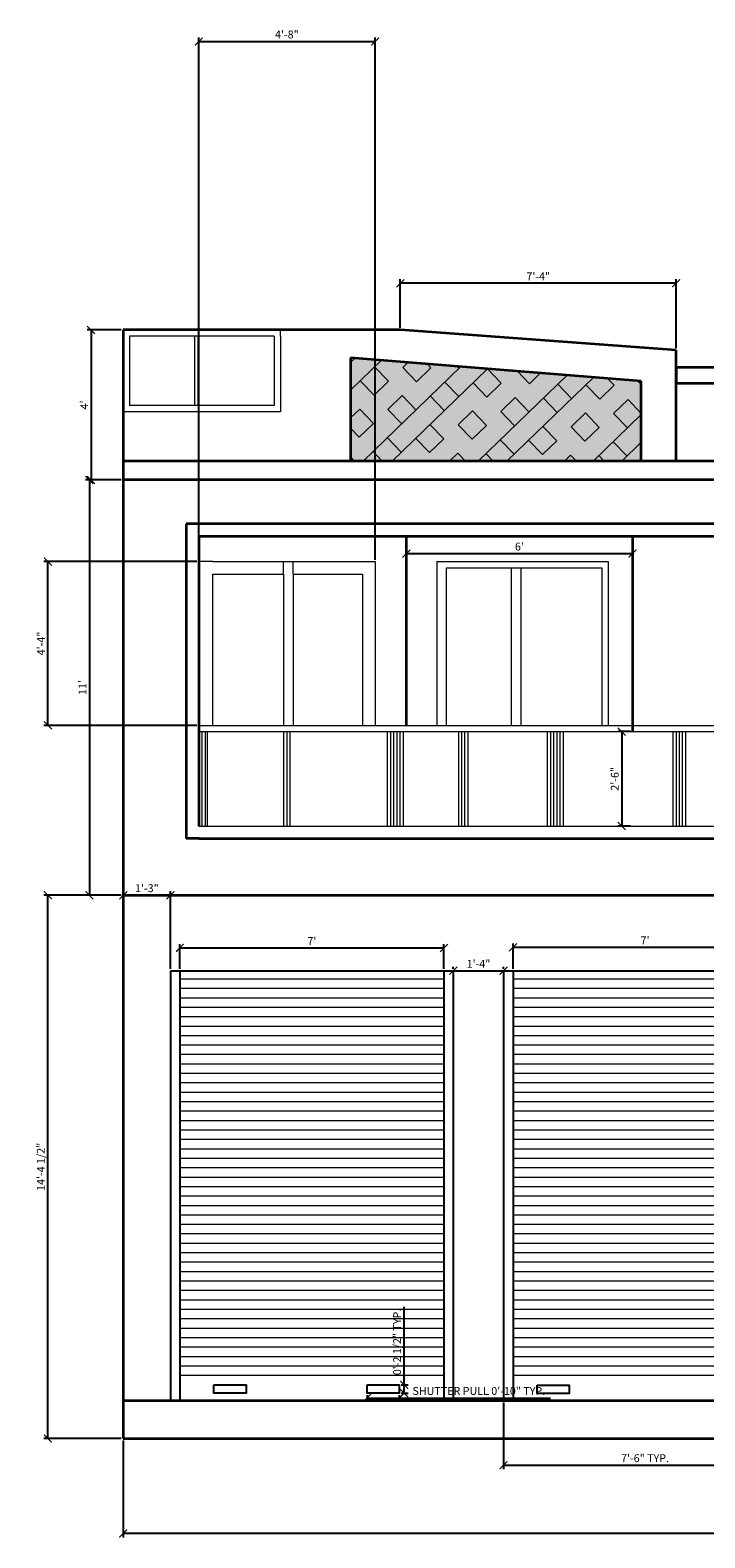
# Model space of a CAD drawing. Units: inches. Extents: x 3122 to 5933, y 1474 to 2995.
# Tile 1 of 12: x 3122 to 3337, y 1583 to 2063. Entities that reach past the tile are written whole.
import ezdxf

# ---------------------------------------------------------------- set-up
doc = ezdxf.new("R2010")
doc.units = ezdxf.units.IN
for name, color, linetype, lineweight in [('A-ANNO-DIMS', 2, 'Continuous', 18), ('A-ELEV', 7, 'Continuous', 35), ('A-ELEV-DOOR', 4, 'Continuous', 25), ('A-ELEV-GLAZ', 4, 'Continuous', 18), ('A-ELEV-PATT', 8, 'Continuous', 13), ('A-ELEV-RAIL', 7, 'Continuous', 18)]:
    doc.layers.add(name, color=color, linetype=linetype, lineweight=lineweight)
doc.styles.get("Standard").update_dxf_attribs({"font": 'arial.ttf'})
doc.dimstyles.new('ISO-25', dxfattribs={"dimtxt": 2.5, "dimasz": 2.5, "dimexe": 1.25, "dimexo": 0.625, "dimtad": 1, "dimdec": 0, "dimlunit": 3, "dimtxsty": 'Standard', "dimblk": 'ARCHTICK', "dimcen": 2.5, "dimadec": 0, "dimazin": 0, "dimtfac": 1, "dimtdec": 0, "dimtmove": 0, "dimatfit": 3, "dimfxl": 1, "dimarcsym": 0})

# ---------------------------------------------------------------- blocks, each defined once
blk = doc.blocks.new('_ArchTick')
at = {"color": 0, "linetype": 'ByBlock', "const_width": 0.15}
blk.add_lwpolyline([(-0.5, -0.5), (0.5, 0.5)], dxfattribs=at)
blk = doc.blocks.new('*D2')
at = {"layer": 'A-ANNO-DIMS', "color": 0, "lineweight": -2, "transparency": 16777216}
for p, q in [((3241.71, 1900.94), (3241.71, 1894.91)), ((3313.71, 1900.94), (3313.71, 1894.91)), ((3241.71, 1896.16), (3313.71, 1896.16))]:
    blk.add_line(p, q, dxfattribs=at)
at = {"layer": 'Defpoints', "color": 0, "transparency": 16777216}
for p in [(3241.71, 1901.56), (3313.71, 1901.56), (3313.71, 1896.16)]:
    blk.add_point(p, dxfattribs=at)
at = {"layer": 'A-ANNO-DIMS', "color": 0, "lineweight": -2, "transparency": 16777216, "xscale": 2.5, "yscale": 2.5, "zscale": 2.5, "rotation": 180}
blk.add_blockref('_ArchTick', (3241.71, 1896.16), dxfattribs=at)
at = {"layer": 'A-ANNO-DIMS', "color": 0, "lineweight": -2, "transparency": 16777216, "xscale": 2.5, "yscale": 2.5, "zscale": 2.5}
blk.add_blockref('_ArchTick', (3313.71, 1896.16), dxfattribs=at)
at = {"layer": 'A-ANNO-DIMS', "color": 0, "transparency": 16777216, "insert": (3277.71, 1898.06), "char_height": 2.5, "attachment_point": 5}
blk.add_mtext("6'", dxfattribs=at)
blk = doc.blocks.new('*D7')
at = {"layer": 'A-ANNO-DIMS', "color": 0, "lineweight": -2, "transparency": 16777216}
for p, q in [((3151.05, 1967.24), (3140.16, 1967.24)), ((3141.41, 1967.24), (3141.41, 1919.56)), ((3151.05, 1919.56), (3140.16, 1919.56))]:
    blk.add_line(p, q, dxfattribs=at)
at = {"layer": 'Defpoints', "color": 0, "transparency": 16777216}
for p in [(3151.68, 1967.24), (3141.41, 1919.56), (3151.68, 1919.56)]:
    blk.add_point(p, dxfattribs=at)
at = {"layer": 'A-ANNO-DIMS', "color": 0, "lineweight": -2, "transparency": 16777216, "xscale": 2.5, "yscale": 2.5, "zscale": 2.5}
for p, rotation in [((3141.41, 1967.24), 90), ((3141.41, 1919.56), 270)]:
    blk.add_blockref('_ArchTick', p, dxfattribs=dict(at, rotation=rotation))
at = {"layer": 'A-ANNO-DIMS', "color": 0, "transparency": 16777216, "insert": (3139.53, 1943.4), "char_height": 2.5, "attachment_point": 5, "rotation": 90}
blk.add_mtext("4'", dxfattribs=at)
blk = doc.blocks.new('*D8')
at = {"layer": 'A-ANNO-DIMS', "color": 0, "lineweight": -2, "transparency": 16777216}
for p, q in [((3151.05, 1919.56), (3139.65, 1919.56)), ((3140.9, 1919.56), (3140.9, 1787.56)), ((3151.05, 1787.56), (3139.65, 1787.56))]:
    blk.add_line(p, q, dxfattribs=at)
at = {"layer": 'Defpoints', "color": 0, "transparency": 16777216}
for p in [(3151.68, 1919.56), (3140.9, 1787.56), (3151.68, 1787.56)]:
    blk.add_point(p, dxfattribs=at)
at = {"layer": 'A-ANNO-DIMS', "color": 0, "lineweight": -2, "transparency": 16777216, "xscale": 2.5, "yscale": 2.5, "zscale": 2.5}
for p, rotation in [((3140.9, 1919.56), 90), ((3140.9, 1787.56), 270)]:
    blk.add_blockref('_ArchTick', p, dxfattribs=dict(at, rotation=rotation))
at = {"layer": 'A-ANNO-DIMS', "color": 0, "transparency": 16777216, "insert": (3139.02, 1853.56), "char_height": 2.5, "attachment_point": 5, "rotation": 90}
blk.add_mtext("11'", dxfattribs=at)
blk = doc.blocks.new('*D9')
at = {"layer": 'A-ANNO-DIMS', "color": 0, "lineweight": -2, "transparency": 16777216}
for p, q in [((3169.68, 1764.19), (3169.68, 1772.06)), ((3169.68, 1770.81), (3253.68, 1770.81)), ((3253.68, 1764.19), (3253.68, 1772.06))]:
    blk.add_line(p, q, dxfattribs=at)
at = {"layer": 'Defpoints', "color": 0, "transparency": 16777216}
for p in [(3253.68, 1770.81), (3169.68, 1763.56), (3253.68, 1763.56)]:
    blk.add_point(p, dxfattribs=at)
at = {"layer": 'A-ANNO-DIMS', "color": 0, "lineweight": -2, "transparency": 16777216, "xscale": 2.5, "yscale": 2.5, "zscale": 2.5, "rotation": 180}
blk.add_blockref('_ArchTick', (3169.68, 1770.81), dxfattribs=at)
at = {"layer": 'A-ANNO-DIMS', "color": 0, "lineweight": -2, "transparency": 16777216, "xscale": 2.5, "yscale": 2.5, "zscale": 2.5}
blk.add_blockref('_ArchTick', (3253.68, 1770.81), dxfattribs=at)
at = {"layer": 'A-ANNO-DIMS', "color": 0, "transparency": 16777216, "insert": (3211.68, 1772.68), "char_height": 2.5, "attachment_point": 5}
blk.add_mtext("7'", dxfattribs=at)
blk = doc.blocks.new('*D10')
at = {"layer": 'A-ANNO-DIMS', "color": 0, "lineweight": -2, "transparency": 16777216}
for p, q in [((3275.68, 1764.19), (3275.68, 1772.26)), ((3275.68, 1771.01), (3359.68, 1771.01)), ((3359.68, 1764.19), (3359.68, 1772.26))]:
    blk.add_line(p, q, dxfattribs=at)
at = {"layer": 'Defpoints', "color": 0, "transparency": 16777216}
for p in [(3359.68, 1771.01), (3275.68, 1763.56), (3359.68, 1763.56)]:
    blk.add_point(p, dxfattribs=at)
at = {"layer": 'A-ANNO-DIMS', "color": 0, "lineweight": -2, "transparency": 16777216, "xscale": 2.5, "yscale": 2.5, "zscale": 2.5, "rotation": 180}
blk.add_blockref('_ArchTick', (3275.68, 1771.01), dxfattribs=at)
at = {"layer": 'A-ANNO-DIMS', "color": 0, "lineweight": -2, "transparency": 16777216, "xscale": 2.5, "yscale": 2.5, "zscale": 2.5}
blk.add_blockref('_ArchTick', (3359.68, 1771.01), dxfattribs=at)
at = {"layer": 'A-ANNO-DIMS', "color": 0, "transparency": 16777216, "insert": (3317.68, 1772.89), "char_height": 2.5, "attachment_point": 5}
blk.add_mtext("7'", dxfattribs=at)
blk = doc.blocks.new('*D11')
at = {"layer": 'A-ANNO-DIMS', "color": 0, "lineweight": -2, "transparency": 16777216}
for p, q in [((3256.68, 1764.19), (3256.68, 1764.81)), ((3256.68, 1763.56), (3272.68, 1763.56)), ((3272.68, 1764.19), (3272.68, 1764.81))]:
    blk.add_line(p, q, dxfattribs=at)
at = {"layer": 'Defpoints', "color": 0, "transparency": 16777216}
for p in [(3256.68, 1763.56), (3272.68, 1763.56), (3272.68, 1763.56)]:
    blk.add_point(p, dxfattribs=at)
at = {"layer": 'A-ANNO-DIMS', "color": 0, "lineweight": -2, "transparency": 16777216, "xscale": 2.5, "yscale": 2.5, "zscale": 2.5, "rotation": 180}
blk.add_blockref('_ArchTick', (3256.68, 1763.56), dxfattribs=at)
at = {"layer": 'A-ANNO-DIMS', "color": 0, "lineweight": -2, "transparency": 16777216, "xscale": 2.5, "yscale": 2.5, "zscale": 2.5}
blk.add_blockref('_ArchTick', (3272.68, 1763.56), dxfattribs=at)
at = {"layer": 'A-ANNO-DIMS', "color": 0, "transparency": 16777216, "insert": (3264.68, 1765.44), "char_height": 2.5, "attachment_point": 5}
blk.add_mtext('1\'-4"', dxfattribs=at)
blk = doc.blocks.new('*D13')
at = {"layer": 'A-ANNO-DIMS', "color": 0, "lineweight": -2, "transparency": 16777216}
for p, q in [((3151.68, 1614.29), (3151.68, 1583.45)), ((3535.57, 1614.29), (3535.57, 1583.45)), ((3535.57, 1584.7), (3151.68, 1584.7))]:
    blk.add_line(p, q, dxfattribs=at)
at = {"layer": 'Defpoints', "color": 0, "transparency": 16777216}
for p in [(3151.68, 1614.92), (3535.57, 1614.92), (3151.68, 1584.7)]:
    blk.add_point(p, dxfattribs=at)
at = {"layer": 'A-ANNO-DIMS', "color": 0, "lineweight": -2, "transparency": 16777216, "xscale": 2.5, "yscale": 2.5, "zscale": 2.5, "rotation": 180}
blk.add_blockref('_ArchTick', (3151.68, 1584.7), dxfattribs=at)
at = {"layer": 'A-ANNO-DIMS', "color": 0, "lineweight": -2, "transparency": 16777216, "xscale": 2.5, "yscale": 2.5, "zscale": 2.5}
blk.add_blockref('_ArchTick', (3535.57, 1584.7), dxfattribs=at)
at = {"layer": 'A-ANNO-DIMS', "color": 0, "transparency": 16777216, "insert": (3343.62, 1586.6), "char_height": 2.5, "attachment_point": 5}
blk.add_mtext("32'", dxfattribs=at)
blk = doc.blocks.new('*D15')
at = {"layer": 'A-ANNO-DIMS', "color": 0, "lineweight": -2, "transparency": 16777216}
for p, q in [((3239.82, 1967.87), (3239.82, 1983.33)), ((3327.58, 1982.08), (3239.82, 1982.08)), ((3327.58, 1961.4), (3327.58, 1983.33))]:
    blk.add_line(p, q, dxfattribs=at)
at = {"layer": 'Defpoints', "color": 0, "transparency": 16777216}
for p in [(3239.82, 1982.08), (3239.82, 1967.24), (3327.58, 1960.78)]:
    blk.add_point(p, dxfattribs=at)
at = {"layer": 'A-ANNO-DIMS', "color": 0, "lineweight": -2, "transparency": 16777216, "xscale": 2.5, "yscale": 2.5, "zscale": 2.5, "rotation": 180}
blk.add_blockref('_ArchTick', (3239.82, 1982.08), dxfattribs=at)
at = {"layer": 'A-ANNO-DIMS', "color": 0, "lineweight": -2, "transparency": 16777216, "xscale": 2.5, "yscale": 2.5, "zscale": 2.5}
blk.add_blockref('_ArchTick', (3327.58, 1982.08), dxfattribs=at)
at = {"layer": 'A-ANNO-DIMS', "color": 0, "transparency": 16777216, "insert": (3283.7, 1983.96), "char_height": 2.5, "attachment_point": 5}
blk.add_mtext('7\'-4"', dxfattribs=at)
blk = doc.blocks.new('*D19')
at = {"layer": 'A-ANNO-DIMS', "color": 0, "lineweight": -2, "transparency": 16777216}
for p, q in [((3313.08, 1839.56), (3309.02, 1839.56)), ((3310.27, 1839.56), (3310.27, 1809.56)), ((3313.08, 1809.56), (3309.02, 1809.56))]:
    blk.add_line(p, q, dxfattribs=at)
at = {"layer": 'Defpoints', "color": 0, "transparency": 16777216}
for p in [(3313.71, 1839.56), (3310.27, 1809.56), (3313.71, 1809.56)]:
    blk.add_point(p, dxfattribs=at)
at = {"layer": 'A-ANNO-DIMS', "color": 0, "lineweight": -2, "transparency": 16777216, "xscale": 2.5, "yscale": 2.5, "zscale": 2.5}
for p, rotation in [((3310.27, 1839.56), 90), ((3310.27, 1809.56), 270)]:
    blk.add_blockref('_ArchTick', p, dxfattribs=dict(at, rotation=rotation))
at = {"layer": 'A-ANNO-DIMS', "color": 0, "transparency": 16777216, "insert": (3308.37, 1824.56), "char_height": 2.5, "attachment_point": 5, "rotation": 90}
blk.add_mtext('2\'-6"', dxfattribs=at)
blk = doc.blocks.new('*D20')
at = {"layer": 'A-ANNO-DIMS', "color": 0, "lineweight": -2, "transparency": 16777216}
for p, q in [((3151.68, 1764.19), (3151.68, 1788.81)), ((3166.68, 1787.56), (3151.68, 1787.56)), ((3166.68, 1764.19), (3166.68, 1788.81))]:
    blk.add_line(p, q, dxfattribs=at)
at = {"layer": 'Defpoints', "color": 0, "transparency": 16777216}
for p in [(3151.68, 1787.56), (3151.68, 1763.56), (3166.68, 1763.56)]:
    blk.add_point(p, dxfattribs=at)
at = {"layer": 'A-ANNO-DIMS', "color": 0, "lineweight": -2, "transparency": 16777216, "xscale": 2.5, "yscale": 2.5, "zscale": 2.5, "rotation": 180}
blk.add_blockref('_ArchTick', (3151.68, 1787.56), dxfattribs=at)
at = {"layer": 'A-ANNO-DIMS', "color": 0, "lineweight": -2, "transparency": 16777216, "xscale": 2.5, "yscale": 2.5, "zscale": 2.5}
blk.add_blockref('_ArchTick', (3166.68, 1787.56), dxfattribs=at)
at = {"layer": 'A-ANNO-DIMS', "color": 0, "transparency": 16777216, "insert": (3159.18, 1789.47), "char_height": 2.5, "attachment_point": 5}
blk.add_mtext('1\'-3"', dxfattribs=at)
blk = doc.blocks.new('SHUTTER-FRAME-84-ELEV')
for p, q in [((0, 136.64), (0, 0)), ((0, 136.64), (90, 136.64)), ((3, 136.64), (3, 0)), ((87, 136.64), (87, 0)), ((90, 136.64), (90, 0))]:
    blk.add_line(p, q)
blk = doc.blocks.new('SHUTTER-LIFT-PULL')
blk.add_lwpolyline([(0, 2.63), (10.24, 2.63), (10.24, 0), (0, 0)], close=True)
blk = doc.blocks.new('*D88')
at = {"layer": 'A-ANNO-DIMS', "color": 0, "lineweight": -2, "transparency": 16777216}
for p, q in [((3229.25, 1628.67), (3229.25, 1626.51)), ((3229.25, 1627.76), (3239.49, 1627.76)), ((3239.49, 1628.67), (3239.49, 1626.51)), ((3239.49, 1627.76), (3287.58, 1627.76))]:
    blk.add_line(p, q, dxfattribs=at)
at = {"layer": 'Defpoints', "color": 0, "transparency": 16777216}
for p in [(3229.25, 1629.3), (3239.49, 1629.3), (3239.49, 1627.76)]:
    blk.add_point(p, dxfattribs=at)
at = {"layer": 'A-ANNO-DIMS', "color": 0, "lineweight": -2, "transparency": 16777216, "xscale": 2.5, "yscale": 2.5, "zscale": 2.5, "rotation": 180}
blk.add_blockref('_ArchTick', (3229.25, 1627.76), dxfattribs=at)
at = {"layer": 'A-ANNO-DIMS', "color": 0, "lineweight": -2, "transparency": 16777216, "xscale": 2.5, "yscale": 2.5, "zscale": 2.5}
blk.add_blockref('_ArchTick', (3239.49, 1627.76), dxfattribs=at)
at = {"layer": 'A-ANNO-DIMS', "color": 0, "transparency": 16777216, "insert": (3264.79, 1629.68), "char_height": 2.5, "attachment_point": 5}
blk.add_mtext('SHUTTER PULL 0\'-10" TYP.', dxfattribs=at)
blk = doc.blocks.new('*D89')
at = {"layer": 'A-ANNO-DIMS', "color": 0, "lineweight": -2, "transparency": 16777216}
for p, q in [((3241.03, 1631.93), (3241.03, 1656.74)), ((3240.12, 1631.93), (3242.28, 1631.93)), ((3241.03, 1629.3), (3241.03, 1631.93)), ((3240.12, 1629.3), (3242.28, 1629.3))]:
    blk.add_line(p, q, dxfattribs=at)
at = {"layer": 'Defpoints', "color": 0, "transparency": 16777216}
for p in [(3239.49, 1631.93), (3241.03, 1631.93), (3239.49, 1629.3)]:
    blk.add_point(p, dxfattribs=at)
at = {"layer": 'A-ANNO-DIMS', "color": 0, "lineweight": -2, "transparency": 16777216, "xscale": 2.5, "yscale": 2.5, "zscale": 2.5}
for p, rotation in [((3241.03, 1631.93), 90), ((3241.03, 1629.3), 270)]:
    blk.add_blockref('_ArchTick', p, dxfattribs=dict(at, rotation=rotation))
at = {"layer": 'A-ANNO-DIMS', "color": 0, "transparency": 16777216, "insert": (3239.11, 1645.59), "char_height": 2.5, "attachment_point": 5, "rotation": 90}
blk.add_mtext('0\'-2 1/2" TYP.', dxfattribs=at)
blk = doc.blocks.new('*D91')
at = {"layer": 'A-ANNO-DIMS', "color": 0, "lineweight": -2, "transparency": 16777216}
for p, q in [((3272.68, 1626.29), (3272.68, 1605.17)), ((3362.68, 1626.29), (3362.68, 1605.17)), ((3272.68, 1606.42), (3362.68, 1606.42))]:
    blk.add_line(p, q, dxfattribs=at)
at = {"layer": 'Defpoints', "color": 0, "transparency": 16777216}
for p in [(3272.68, 1626.92), (3362.68, 1626.92), (3362.68, 1606.42)]:
    blk.add_point(p, dxfattribs=at)
at = {"layer": 'A-ANNO-DIMS', "color": 0, "lineweight": -2, "transparency": 16777216, "xscale": 2.5, "yscale": 2.5, "zscale": 2.5, "rotation": 180}
blk.add_blockref('_ArchTick', (3272.68, 1606.42), dxfattribs=at)
at = {"layer": 'A-ANNO-DIMS', "color": 0, "lineweight": -2, "transparency": 16777216, "xscale": 2.5, "yscale": 2.5, "zscale": 2.5}
blk.add_blockref('_ArchTick', (3362.68, 1606.42), dxfattribs=at)
at = {"layer": 'A-ANNO-DIMS', "color": 0, "transparency": 16777216, "insert": (3317.68, 1608.32), "char_height": 2.5, "attachment_point": 5}
blk.add_mtext('7\'-6" TYP.', dxfattribs=at)
blk = doc.blocks.new('*D118')
at = {"layer": 'A-ANNO-DIMS', "color": 0, "lineweight": -2, "transparency": 16777216}
for p, q in [((3151.05, 1787.56), (3126.43, 1787.56)), ((3127.68, 1614.92), (3127.68, 1787.56)), ((3151.05, 1614.92), (3126.43, 1614.92))]:
    blk.add_line(p, q, dxfattribs=at)
at = {"layer": 'Defpoints', "color": 0, "transparency": 16777216}
for p in [(3127.68, 1787.56), (3151.68, 1787.56), (3151.68, 1614.92)]:
    blk.add_point(p, dxfattribs=at)
at = {"layer": 'A-ANNO-DIMS', "color": 0, "lineweight": -2, "transparency": 16777216, "xscale": 2.5, "yscale": 2.5, "zscale": 2.5}
for p, rotation in [((3127.68, 1787.56), 90), ((3127.68, 1614.92), 270)]:
    blk.add_blockref('_ArchTick', p, dxfattribs=dict(at, rotation=rotation))
at = {"layer": 'A-ANNO-DIMS', "color": 0, "transparency": 16777216, "insert": (3125.76, 1701.24), "char_height": 2.5, "attachment_point": 5, "rotation": 90}
blk.add_mtext('14\'-4 1/2"', dxfattribs=at)
blk = doc.blocks.new('*D123')
at = {"layer": 'A-ANNO-DIMS', "color": 0, "lineweight": -2, "transparency": 16777216}
for p, q in [((3175.68, 1894.22), (3175.68, 2060.17)), ((3175.68, 2058.92), (3231.77, 2058.92)), ((3231.77, 1894.22), (3231.77, 2060.17))]:
    blk.add_line(p, q, dxfattribs=at)
at = {"layer": 'Defpoints', "color": 0, "transparency": 16777216}
for p in [(3231.77, 2058.92), (3175.68, 1893.59), (3231.77, 1893.59)]:
    blk.add_point(p, dxfattribs=at)
at = {"layer": 'A-ANNO-DIMS', "color": 0, "lineweight": -2, "transparency": 16777216, "xscale": 2.5, "yscale": 2.5, "zscale": 2.5, "rotation": 180}
blk.add_blockref('_ArchTick', (3175.68, 2058.92), dxfattribs=at)
at = {"layer": 'A-ANNO-DIMS', "color": 0, "lineweight": -2, "transparency": 16777216, "xscale": 2.5, "yscale": 2.5, "zscale": 2.5}
blk.add_blockref('_ArchTick', (3231.77, 2058.92), dxfattribs=at)
at = {"layer": 'A-ANNO-DIMS', "color": 0, "transparency": 16777216, "insert": (3203.72, 2060.82), "char_height": 2.5, "attachment_point": 5}
blk.add_mtext('4\'-8"', dxfattribs=at)
blk = doc.blocks.new('*D124')
at = {"layer": 'A-ANNO-DIMS', "color": 0, "lineweight": -2, "transparency": 16777216}
for p, q in [((3175.05, 1893.59), (3126.43, 1893.59)), ((3127.68, 1841.56), (3127.68, 1893.59)), ((3175.05, 1841.56), (3126.43, 1841.56))]:
    blk.add_line(p, q, dxfattribs=at)
at = {"layer": 'Defpoints', "color": 0, "transparency": 16777216}
for p in [(3127.68, 1893.59), (3175.68, 1893.59), (3175.68, 1841.56)]:
    blk.add_point(p, dxfattribs=at)
at = {"layer": 'A-ANNO-DIMS', "color": 0, "lineweight": -2, "transparency": 16777216, "xscale": 2.5, "yscale": 2.5, "zscale": 2.5}
for p, rotation in [((3127.68, 1893.59), 90), ((3127.68, 1841.56), 270)]:
    blk.add_blockref('_ArchTick', p, dxfattribs=dict(at, rotation=rotation))
at = {"layer": 'A-ANNO-DIMS', "color": 0, "transparency": 16777216, "insert": (3125.8, 1867.58), "char_height": 2.5, "attachment_point": 5, "rotation": 90}
blk.add_mtext('4\'-4"', dxfattribs=at)

msp = doc.modelspace()

# ---------------------------------------------------------------- hatches: boundary and pattern name
at = {"layer": 'A-ELEV-PATT'}
h = msp.add_hatch(dxfattribs=at)
h.set_pattern_fill('BOX', color=256, angle=134)
h.paths.add_polyline_path([(3316.49, 1951), (3223.95, 1958.38), (3223.95, 1925.56), (3316.49, 1925.56)])
h = msp.add_hatch(dxfattribs=at)
h.set_pattern_fill('BOX', color=256, scale=0.1, angle=86)
h.paths.add_polyline_path([(3316.49, 1951), (3223.95, 1958.38), (3223.95, 1925.56), (3316.49, 1925.56)])
h = msp.add_hatch(dxfattribs=at)
h.set_pattern_fill('ANSI31', color=256, scale=0.944882, angle=-45, style=0)
h.paths.add_polyline_path([(3169.68, 1634.07), (3253.68, 1634.07), (3253.68, 1763.05), (3169.68, 1763.05)])
h = msp.add_hatch(dxfattribs=at)
h.set_pattern_fill('ANSI31', color=256, scale=0.944882, angle=-45, style=0)
h.paths.add_polyline_path([(3275.68, 1634.07), (3359.68, 1634.07), (3359.68, 1763.05), (3275.68, 1763.05)])

# ---------------------------------------------------------------- linework, layer by layer
at = {"layer": 'A-ELEV'}
for p, q in [((3239.82, 1967.24), (3151.68, 1967.24)), ((3151.68, 1967.24), (3151.68, 1919.56)), ((3327.58, 1960.78), (3239.82, 1967.24)), ((3327.58, 1925.56), (3327.58, 1960.78)), ((3316.49, 1951), (3223.95, 1958.38)), ((3223.95, 1958.38), (3223.95, 1925.56)), ((3353.11, 1955.27), (3327.58, 1955.27)), ((3327.58, 1955.27), (3327.58, 1950.27)), ((3316.49, 1925.56), (3316.49, 1951)), ((3327.58, 1950.27), (3353.11, 1950.27)), ((3529.68, 1925.56), (3151.68, 1925.56)), ((3535.57, 1919.56), (3151.68, 1919.56)), ((3151.68, 1919.56), (3151.68, 1787.56)), ((3535.57, 1905.56), (3171.68, 1905.56)), ((3171.68, 1905.56), (3171.68, 1805.56)), ((3535.57, 1901.56), (3175.68, 1901.56)), ((3175.68, 1901.56), (3175.68, 1809.56)), ((3241.71, 1901.56), (3241.71, 1841.56)), ((3313.71, 1901.56), (3313.71, 1839.56)), ((3175.68, 1805.56), (3171.68, 1805.56)), ((3175.68, 1805.56), (3535.57, 1805.56)), ((3151.68, 1787.56), (3535.57, 1787.56)), ((3151.68, 1787.56), (3151.68, 1614.92)), ((3151.68, 1626.92), (3535.57, 1626.92)), ((3151.68, 1614.92), (3535.57, 1614.92))]:
    msp.add_line(p, q, dxfattribs=at)
at = {"layer": 'A-ELEV-GLAZ'}
for p, q in [((3199.68, 1965.24), (3153.68, 1965.24)), ((3153.68, 1965.24), (3153.68, 1943.24)), ((3174.38, 1965.24), (3174.38, 1943.24)), ((3175.38, 1965.24), (3175.38, 1943.24)), ((3199.68, 1965.24), (3199.68, 1943.24)), ((3201.68, 1965.24), (3201.68, 1967.24)), ((3201.68, 1965.24), (3201.68, 1941.24)), ((3201.68, 1941.24), (3151.68, 1941.24)), ((3199.68, 1943.24), (3153.68, 1943.24)), ((3180.18, 1893.59), (3175.68, 1893.59)), ((3180.18, 1893.59), (3231.77, 1893.59)), ((3202.68, 1889.59), (3202.68, 1893.59)), ((3205.68, 1889.59), (3205.68, 1893.59)), ((3231.77, 1893.59), (3231.77, 1841.56)), ((3251.45, 1893.59), (3251.45, 1841.56)), ((3251.45, 1893.59), (3260.61, 1893.59)), ((3260.61, 1893.59), (3305.97, 1893.59)), ((3305.97, 1893.59), (3305.97, 1841.56)), ((3180.18, 1841.56), (3180.18, 1889.59)), ((3180.18, 1889.59), (3202.68, 1889.59)), ((3202.68, 1889.59), (3202.68, 1841.56)), ((3205.68, 1889.59), (3227.77, 1889.59)), ((3205.68, 1889.59), (3205.68, 1841.56)), ((3227.77, 1889.59), (3227.77, 1841.56)), ((3254.45, 1891.59), (3254.45, 1841.56)), ((3254.45, 1891.59), (3260.61, 1891.59)), ((3260.61, 1891.59), (3303.97, 1891.59)), ((3275.11, 1891.59), (3275.11, 1841.56)), ((3278.11, 1891.59), (3278.11, 1841.56)), ((3303.97, 1891.59), (3303.97, 1841.56))]:
    msp.add_line(p, q, dxfattribs=at)
at = {"layer": 'A-ELEV-RAIL'}
for p, q in [((3175.68, 1841.56), (3535.57, 1841.56)), ((3175.68, 1839.56), (3235.68, 1839.56)), ((3176.68, 1839.56), (3176.68, 1809.56)), ((3177.68, 1839.56), (3177.68, 1809.56)), ((3178.37, 1839.56), (3178.37, 1809.56)), ((3202.68, 1839.56), (3202.68, 1809.56)), ((3203.68, 1839.56), (3203.68, 1809.56)), ((3204.68, 1839.56), (3204.68, 1809.56)), ((3235.68, 1839.56), (3535.57, 1839.56)), ((3235.68, 1839.56), (3235.68, 1809.56)), ((3236.68, 1839.56), (3236.68, 1809.56)), ((3237.68, 1839.56), (3237.68, 1809.56)), ((3238.68, 1839.56), (3238.68, 1809.56)), ((3239.68, 1839.56), (3239.68, 1809.56)), ((3240.68, 1839.56), (3240.68, 1809.56)), ((3258.28, 1839.56), (3258.28, 1809.56)), ((3259.28, 1839.56), (3259.28, 1809.56)), ((3260.28, 1839.56), (3260.28, 1809.56)), ((3261.28, 1839.56), (3261.28, 1809.56)), ((3286.58, 1839.56), (3286.58, 1809.56)), ((3287.58, 1839.56), (3287.58, 1809.56)), ((3288.58, 1839.56), (3288.58, 1809.56)), ((3289.58, 1839.56), (3289.58, 1809.56)), ((3290.58, 1839.56), (3290.58, 1809.56)), ((3291.58, 1839.56), (3291.58, 1809.56)), ((3326.54, 1839.56), (3326.54, 1809.56)), ((3327.54, 1839.56), (3327.54, 1809.56)), ((3328.54, 1839.56), (3328.54, 1809.56)), ((3329.54, 1839.56), (3329.54, 1809.56)), ((3330.54, 1839.56), (3330.54, 1809.56)), ((3175.68, 1809.56), (3235.68, 1809.56)), ((3235.68, 1809.56), (3240.68, 1809.56)), ((3240.68, 1809.56), (3535.57, 1809.56))]:
    msp.add_line(p, q, dxfattribs=at)

# ---------------------------------------------------------------- block references
at = {"layer": 'A-ELEV-DOOR'}
for name, p in [('SHUTTER-FRAME-84-ELEV', (3166.68, 1626.92)), ('SHUTTER-FRAME-84-ELEV', (3272.68, 1626.92)), ('SHUTTER-LIFT-PULL', (3180.49, 1629.3)), ('SHUTTER-LIFT-PULL', (3229.25, 1629.3)), ('SHUTTER-LIFT-PULL', (3283.33, 1629.18))]:
    msp.add_blockref(name, p, dxfattribs=at)

# ---------------------------------------------------------------- dimensions: what is measured, and where the dimension line sits
at = {"layer": 'A-ANNO-DIMS'}
for base, p1, p2, override, picture, middle in [((3231.77, 2058.92), (3175.68, 1893.59), (3231.77, 1893.59), {"dimdec": 1, "dimlfac": 1, "dimrnd": 0, "dimzin": 1, "dimdsep": 46, "dimlunit": 4, "dimfrac": 2}, '*D123', (3203.72, 2060.82)), ((3239.82, 1982.08), (3327.58, 1960.78), (3239.82, 1967.24), {"dimclrd": 0, "dimclre": 0, "dimclrt": 0}, '*D15', (3283.7, 1983.96)), ((3313.71, 1896.16), (3241.71, 1901.56), (3313.71, 1901.56), {"dimclrd": 0, "dimclre": 0, "dimclrt": 0}, '*D2', (3277.71, 1898.06)), ((3151.68, 1787.56), (3166.68, 1763.56), (3151.68, 1763.56), {"dimclrd": 0, "dimclre": 0, "dimclrt": 0}, '*D20', (3159.18, 1789.47)), ((3253.68, 1770.81), (3169.68, 1763.56), (3253.68, 1763.56), {"dimclrd": 0, "dimclre": 0, "dimclrt": 0}, '*D9', (3211.68, 1772.68)), ((3359.68, 1771.01), (3275.68, 1763.56), (3359.68, 1763.56), {"dimclrd": 0, "dimclre": 0, "dimclrt": 0}, '*D10', (3317.68, 1772.89)), ((3272.68, 1763.56), (3256.68, 1763.56), (3272.68, 1763.56), {"dimclrd": 0, "dimclre": 0, "dimclrt": 0}, '*D11', (3264.68, 1765.44)), ((3151.68, 1584.7), (3535.57, 1614.92), (3151.68, 1614.92), {"dimclrd": 0, "dimclre": 0, "dimclrt": 0}, '*D13', (3343.62, 1586.6))]:
    dim = msp.add_linear_dim(base=base, p1=p1, p2=p2, dimstyle='ISO-25', override=override, dxfattribs=at)
    dim.commit()
    dim.dimension.update_dxf_attribs({"geometry": picture, "text_midpoint": middle})
for base, p1, p2, override, picture, middle in [((3141.41, 1919.56), (3151.68, 1967.24), (3151.68, 1919.56), {"dimclrd": 0, "dimclre": 0, "dimclrt": 0}, '*D7', (3139.53, 1943.4)), ((3140.9, 1787.56), (3151.68, 1919.56), (3151.68, 1787.56), {"dimclrd": 0, "dimclre": 0, "dimclrt": 0}, '*D8', (3139.02, 1853.56)), ((3127.68, 1893.59), (3175.68, 1841.56), (3175.68, 1893.59), {"dimdec": 1, "dimlfac": 1, "dimrnd": 0, "dimzin": 1, "dimdsep": 46, "dimlunit": 4, "dimfrac": 2}, '*D124', (3125.8, 1867.58)), ((3310.27, 1809.56), (3313.71, 1839.56), (3313.71, 1809.56), {"dimclrd": 0, "dimclre": 0, "dimclrt": 0}, '*D19', (3308.37, 1824.56)), ((3127.68, 1787.56), (3151.68, 1614.92), (3151.68, 1787.56), {"dimdec": 1, "dimlfac": 1, "dimrnd": 0, "dimzin": 1, "dimdsep": 46, "dimlunit": 4, "dimfrac": 2}, '*D118', (3125.76, 1701.24))]:
    dim = msp.add_linear_dim(base=base, p1=p1, p2=p2, angle=90, dimstyle='ISO-25', override=override, dxfattribs=at)
    dim.commit()
    dim.dimension.update_dxf_attribs({"geometry": picture, "text_midpoint": middle})
dim = msp.add_linear_dim(base=(3241.03, 1631.93), p1=(3239.49, 1629.3), p2=(3239.49, 1631.93), angle=90, text='<> TYP.', dimstyle='ISO-25', override={"dimdec": 1, "dimlfac": 1, "dimrnd": 0, "dimzin": 1, "dimdsep": 46, "dimlunit": 4, "dimfrac": 2}, dxfattribs=at)
dim.commit()
dim.dimension.update_dxf_attribs({"geometry": '*D89', "text_midpoint": (3239.11, 1645.59)})
for base, p1, p2, text, picture, middle in [((3239.49, 1627.76), (3229.25, 1629.3), (3239.49, 1629.3), 'SHUTTER PULL <> TYP.', '*D88', (3264.79, 1629.68)), ((3362.68, 1606.42), (3272.68, 1626.92), (3362.68, 1626.92), '<> TYP.', '*D91', (3317.68, 1608.32))]:
    dim = msp.add_linear_dim(base=base, p1=p1, p2=p2, text=text, dimstyle='ISO-25', override={"dimdec": 1, "dimlfac": 1, "dimrnd": 0, "dimzin": 1, "dimdsep": 46, "dimlunit": 4, "dimfrac": 2}, dxfattribs=at)
    dim.commit()
    dim.dimension.update_dxf_attribs({"geometry": picture, "text_midpoint": middle})

doc.saveas('drawing.dxf')
